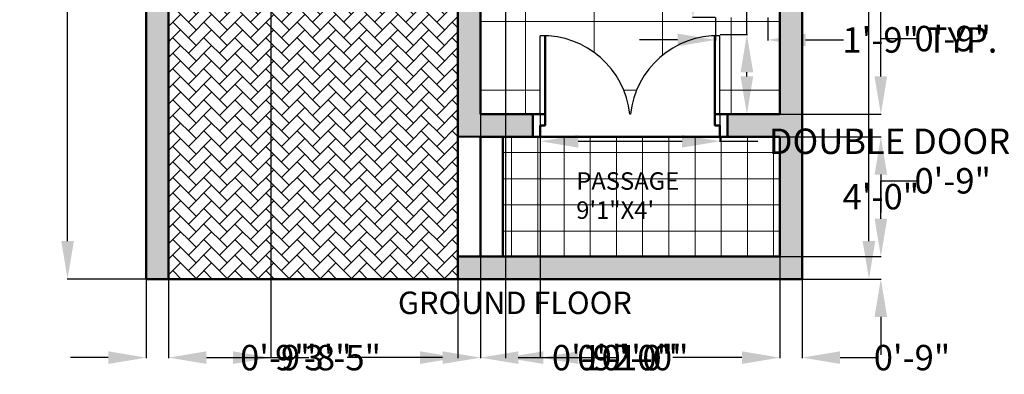
# Model space of a CAD drawing. Units: inches. Extents: x 26 to 14419, y 2 to 3479.
# Tile 1 of 9: x 13608 to 14003, y 2804 to 2946. Entities that reach past the tile are written whole.
import ezdxf

# ---------------------------------------------------------------- set-up
doc = ezdxf.new("R2010")
doc.units = ezdxf.units.IN
doc.header["$MEASUREMENT"] = 0
for name, color, linetype, lineweight in [('A-ANNO-DIMS', 2, 'Continuous', 18), ('A-ANNO-TEXT', 7, 'Continuous', 25), ('A-AREA-IDEN', 7, 'Continuous', 18), ('A-DOOR', 4, 'Continuous', 25), ('A-FLOR-PATT', 252, 'Continuous', 13), ('A-FURN', 8, 'Continuous', 18), ('A-WALL', 7, 'Continuous', 50)]:
    doc.layers.add(name, color=color, linetype=linetype, lineweight=lineweight)
doc.styles.get("Standard").update_dxf_attribs({"font": 'arial.ttf'})
doc.dimstyles.get("Standard").update_dxf_attribs({"dimtxt": 10.18, "dimasz": 15.18, "dimexe": 0.18, "dimexo": 0.0625, "dimgap": 0.09, "dimtad": 0, "dimtih": 1, "dimtoh": 1, "dimdec": 0, "dimzin": 0, "dimdsep": 46, "dimlunit": 3, "dimtxsty": 'Standard', "dimcen": 0.09, "dimadec": 0, "dimazin": 0, "dimtfac": 1, "dimtdec": 0, "dimtofl": 0, "dimtmove": 0, "dimatfit": 3, "dimfxl": 1, "dimtolj": 1, "dimtzin": 0, "dimarcsym": 0})

# ---------------------------------------------------------------- blocks, each defined once
blk = doc.blocks.new('*D7')
at = {"layer": 'A-ANNO-DIMS', "color": 0, "lineweight": -2, "transparency": 16777216}
for p, q in [((13922.15, 3432), (13949, 3432)), ((13948.82, 3416.82), (13948.82, 3142.28)), ((13948.82, 2857.18), (13948.82, 3131.71)), ((13922.15, 2842), (13949, 2842))]:
    blk.add_line(p, q, dxfattribs=at)
at = {"layer": 'A-ANNO-DIMS', "color": 0, "transparency": 16777216}
for points in [[(13946.29, 3416.82), (13951.35, 3416.82), (13948.82, 3432)], [(13946.29, 2857.18), (13951.35, 2857.18), (13948.82, 2842)]]:
    blk.add_solid(points, dxfattribs=at)
at = {"layer": 'Defpoints', "color": 0, "transparency": 16777216}
for p in [(13922.09, 3432), (13922.09, 2842), (13948.82, 2842)]:
    blk.add_point(p, dxfattribs=at)
at = {"layer": 'A-ANNO-DIMS', "color": 0, "transparency": 16777216, "insert": (13948.82, 3137), "char_height": 10.18, "attachment_point": 5}
blk.add_mtext('\\A1;49\'-2"', dxfattribs=at)
blk = doc.blocks.new('DOOR-DOUBLE')
for p, q in [((0, 0), (0, 31.5)), ((72, 0), (72, 31.5)), ((36.16, 0), (35.84, 0))]:
    blk.add_line(p, q)
for centre, start, end in [((1, -3.5), 5.7368, 91.6366), ((71, -3.5), 88.3634, 174.2632)]:
    blk.add_arc(centre, 35.01, start, end)
blk = doc.blocks.new('*D29')
at = {"layer": 'A-ANNO-DIMS', "color": 0, "lineweight": -2, "transparency": 16777216}
for p, q in [((13817.09, 2907.93), (13817.09, 2897.02)), ((13889.09, 2907.93), (13889.09, 2897.02)), ((13832.27, 2897.2), (13873.91, 2897.2)), ((13889.09, 2897.2), (13904.27, 2897.2))]:
    blk.add_line(p, q, dxfattribs=at)
at = {"layer": 'A-ANNO-DIMS', "color": 0, "transparency": 16777216}
for points in [[(13832.27, 2899.73), (13832.27, 2894.67), (13817.09, 2897.2)], [(13873.91, 2899.73), (13873.91, 2894.67), (13889.09, 2897.2)]]:
    blk.add_solid(points, dxfattribs=at)
at = {"layer": 'Defpoints', "color": 0, "transparency": 16777216}
for p in [(13817.09, 2908), (13889.09, 2908), (13889.09, 2897.2)]:
    blk.add_point(p, dxfattribs=at)
at = {"layer": 'A-ANNO-DIMS', "color": 0, "transparency": 16777216, "insert": (13989.66, 2897.2), "char_height": 10.18, "attachment_point": 5}
blk.add_mtext('\\A1;DOUBLE DOOR 6\'-0" TYP.', dxfattribs=at)
blk = doc.blocks.new('*D30')
at = {"layer": 'A-ANNO-DIMS', "color": 0, "lineweight": -2, "transparency": 16777216}
for p, q in [((13899.89, 2940.02), (13899.89, 2955.2)), ((13899.89, 2955.2), (13915.07, 2955.2)), ((13889.15, 2940.02), (13900.07, 2940.02)), ((13899.89, 2923.18), (13899.89, 2924.84)), ((13889.15, 2908), (13900.07, 2908))]:
    blk.add_line(p, q, dxfattribs=at)
at = {"layer": 'A-ANNO-DIMS', "color": 0, "transparency": 16777216}
for points in [[(13897.36, 2924.84), (13902.42, 2924.84), (13899.89, 2940.02)], [(13897.36, 2923.18), (13902.42, 2923.18), (13899.89, 2908)]]:
    blk.add_solid(points, dxfattribs=at)
at = {"layer": 'Defpoints', "color": 0, "transparency": 16777216}
for p in [(13889.09, 2940.02), (13899.89, 2940.02), (13889.09, 2908)]:
    blk.add_point(p, dxfattribs=at)
at = {"layer": 'A-ANNO-DIMS', "color": 0, "transparency": 16777216, "insert": (13946.27, 2955.2), "char_height": 10.18, "attachment_point": 5}
blk.add_mtext('\\A1;2\'-8" TYP.', dxfattribs=at)
blk = doc.blocks.new('*D31')
at = {"layer": 'A-ANNO-DIMS', "color": 0, "lineweight": -2, "transparency": 16777216}
for p, q in [((13887.2, 3006.75), (13878.09, 3006.75)), ((13878.27, 2991.57), (13878.27, 2982.14)), ((13878.27, 2961.99), (13878.27, 2971.42)), ((13887.2, 2946.81), (13878.09, 2946.81))]:
    blk.add_line(p, q, dxfattribs=at)
at = {"layer": 'A-ANNO-DIMS', "color": 0, "transparency": 16777216}
for points in [[(13875.74, 2991.57), (13880.8, 2991.57), (13878.27, 3006.75)], [(13875.74, 2961.99), (13880.8, 2961.99), (13878.27, 2946.81)]]:
    blk.add_solid(points, dxfattribs=at)
at = {"layer": 'Defpoints', "color": 0, "transparency": 16777216}
for p in [(13887.26, 3006.75), (13878.27, 2946.81), (13887.26, 2946.81)]:
    blk.add_point(p, dxfattribs=at)
at = {"layer": 'A-ANNO-DIMS', "color": 0, "transparency": 16777216, "insert": (13878.27, 2976.78), "char_height": 10.18, "attachment_point": 5}
blk.add_mtext('\\A1;3-SEAT SOFA 5\'-0" TYP.', dxfattribs=at)
blk = doc.blocks.new('*D32')
at = {"layer": 'A-ANNO-DIMS', "color": 0, "lineweight": -2, "transparency": 16777216}
for p, q in [((13887.26, 2946.75), (13887.26, 2937.64)), ((13908.25, 2946.75), (13908.25, 2937.64)), ((13872.08, 2937.82), (13856.9, 2937.82)), ((13923.43, 2937.82), (13938.61, 2937.82))]:
    blk.add_line(p, q, dxfattribs=at)
at = {"layer": 'A-ANNO-DIMS', "color": 0, "transparency": 16777216}
for points in [[(13872.08, 2940.35), (13872.08, 2935.29), (13887.26, 2937.82)], [(13923.43, 2940.35), (13923.43, 2935.29), (13908.25, 2937.82)]]:
    blk.add_solid(points, dxfattribs=at)
at = {"layer": 'Defpoints', "color": 0, "transparency": 16777216}
for p in [(13887.26, 2946.81), (13908.25, 2946.81), (13908.25, 2937.82)]:
    blk.add_point(p, dxfattribs=at)
at = {"layer": 'A-ANNO-DIMS', "color": 0, "transparency": 16777216, "insert": (13969.25, 2937.82), "char_height": 10.18, "attachment_point": 5}
blk.add_mtext('\\A1;1\'-9" TYP.', dxfattribs=at)
blk = doc.blocks.new('*D51')
at = {"layer": 'A-ANNO-DIMS', "color": 0, "lineweight": -2, "transparency": 16777216}
for p, q in [((13659.09, 2841.93), (13659.09, 2810.32)), ((13668.09, 2841.93), (13668.09, 2810.32)), ((13643.91, 2810.5), (13628.73, 2810.5)), ((13683.27, 2810.5), (13698.45, 2810.5))]:
    blk.add_line(p, q, dxfattribs=at)
at = {"layer": 'A-ANNO-DIMS', "color": 0, "transparency": 16777216}
for points in [[(13643.91, 2813.03), (13643.91, 2807.97), (13659.09, 2810.5)], [(13683.27, 2813.03), (13683.27, 2807.97), (13668.09, 2810.5)]]:
    blk.add_solid(points, dxfattribs=at)
at = {"layer": 'Defpoints', "color": 0, "transparency": 16777216}
for p in [(13659.09, 2842), (13668.09, 2842), (13668.09, 2810.5)]:
    blk.add_point(p, dxfattribs=at)
at = {"layer": 'A-ANNO-DIMS', "color": 0, "transparency": 16777216, "insert": (13712.07, 2810.5), "char_height": 10.18, "attachment_point": 5}
blk.add_mtext('\\A1;0\'-9"', dxfattribs=at)
blk = doc.blocks.new('*D52')
at = {"layer": 'A-ANNO-DIMS', "color": 0, "lineweight": -2, "transparency": 16777216}
for p, q in [((13668.09, 2841.93), (13668.09, 2810.32)), ((13784.09, 2841.93), (13784.09, 2810.32)), ((13683.27, 2810.5), (13712.47, 2810.5)), ((13768.91, 2810.5), (13739.71, 2810.5))]:
    blk.add_line(p, q, dxfattribs=at)
at = {"layer": 'A-ANNO-DIMS', "color": 0, "transparency": 16777216}
for points in [[(13683.27, 2813.03), (13683.27, 2807.97), (13668.09, 2810.5)], [(13768.91, 2813.03), (13768.91, 2807.97), (13784.09, 2810.5)]]:
    blk.add_solid(points, dxfattribs=at)
at = {"layer": 'Defpoints', "color": 0, "transparency": 16777216}
for p in [(13668.09, 2842), (13784.09, 2842), (13784.09, 2810.5)]:
    blk.add_point(p, dxfattribs=at)
at = {"layer": 'A-ANNO-DIMS', "color": 0, "transparency": 16777216, "insert": (13726.09, 2810.5), "char_height": 10.18, "attachment_point": 5}
blk.add_mtext('\\A1;9\'-8"', dxfattribs=at)
blk = doc.blocks.new('*D53')
at = {"layer": 'A-ANNO-DIMS', "color": 0, "lineweight": -2, "transparency": 16777216}
for p, q in [((13793.09, 2850.93), (13793.09, 2810.32)), ((13784.09, 2841.93), (13784.09, 2810.32)), ((13768.91, 2810.5), (13753.73, 2810.5)), ((13808.27, 2810.5), (13823.45, 2810.5))]:
    blk.add_line(p, q, dxfattribs=at)
at = {"layer": 'A-ANNO-DIMS', "color": 0, "transparency": 16777216}
for points in [[(13768.91, 2813.03), (13768.91, 2807.97), (13784.09, 2810.5)], [(13808.27, 2813.03), (13808.27, 2807.97), (13793.09, 2810.5)]]:
    blk.add_solid(points, dxfattribs=at)
at = {"layer": 'Defpoints', "color": 0, "transparency": 16777216}
for p in [(13793.09, 2851), (13784.09, 2842), (13793.09, 2810.5)]:
    blk.add_point(p, dxfattribs=at)
at = {"layer": 'A-ANNO-DIMS', "color": 0, "transparency": 16777216, "insert": (13837.07, 2810.5), "char_height": 10.18, "attachment_point": 5}
blk.add_mtext('\\A1;0\'-9"', dxfattribs=at)
blk = doc.blocks.new('*D54')
at = {"layer": 'A-ANNO-DIMS', "color": 0, "lineweight": -2, "transparency": 16777216}
for p, q in [((13793.09, 2850.93), (13793.09, 2810.32)), ((13913.09, 2850.93), (13913.09, 2810.32)), ((13808.27, 2810.5), (13836, 2810.5)), ((13897.91, 2810.5), (13870.19, 2810.5))]:
    blk.add_line(p, q, dxfattribs=at)
at = {"layer": 'A-ANNO-DIMS', "color": 0, "transparency": 16777216}
for points in [[(13808.27, 2813.03), (13808.27, 2807.97), (13793.09, 2810.5)], [(13897.91, 2813.03), (13897.91, 2807.97), (13913.09, 2810.5)]]:
    blk.add_solid(points, dxfattribs=at)
at = {"layer": 'Defpoints', "color": 0, "transparency": 16777216}
for p in [(13793.09, 2851), (13913.09, 2851), (13913.09, 2810.5)]:
    blk.add_point(p, dxfattribs=at)
at = {"layer": 'A-ANNO-DIMS', "color": 0, "transparency": 16777216, "insert": (13853.09, 2810.5), "char_height": 10.18, "attachment_point": 5}
blk.add_mtext('\\A1;10\'-0"', dxfattribs=at)
blk = doc.blocks.new('*D55')
at = {"layer": 'A-ANNO-DIMS', "color": 0, "lineweight": -2, "transparency": 16777216}
for p, q in [((13913.09, 2850.93), (13913.09, 2810.32)), ((13922.09, 2841.93), (13922.09, 2810.32)), ((13897.91, 2810.5), (13882.73, 2810.5)), ((13937.27, 2810.5), (13952.45, 2810.5))]:
    blk.add_line(p, q, dxfattribs=at)
at = {"layer": 'A-ANNO-DIMS', "color": 0, "transparency": 16777216}
for points in [[(13897.91, 2813.03), (13897.91, 2807.97), (13913.09, 2810.5)], [(13937.27, 2813.03), (13937.27, 2807.97), (13922.09, 2810.5)]]:
    blk.add_solid(points, dxfattribs=at)
at = {"layer": 'Defpoints', "color": 0, "transparency": 16777216}
for p in [(13913.09, 2851), (13922.09, 2842), (13922.09, 2810.5)]:
    blk.add_point(p, dxfattribs=at)
at = {"layer": 'A-ANNO-DIMS', "color": 0, "transparency": 16777216, "insert": (13966.07, 2810.5), "char_height": 10.18, "attachment_point": 5}
blk.add_mtext('\\A1;0\'-9"', dxfattribs=at)
blk = doc.blocks.new('*D56')
at = {"layer": 'A-ANNO-DIMS', "color": 0, "lineweight": -2, "transparency": 16777216}
for p, q in [((13668.03, 3076), (13627.41, 3076)), ((13627.59, 3060.82), (13627.59, 2964.28)), ((13627.59, 2857.18), (13627.59, 2953.71)), ((13668.03, 2842), (13627.41, 2842))]:
    blk.add_line(p, q, dxfattribs=at)
at = {"layer": 'A-ANNO-DIMS', "color": 0, "transparency": 16777216}
for points in [[(13625.06, 3060.82), (13630.12, 3060.82), (13627.59, 3076)], [(13625.06, 2857.18), (13630.12, 2857.18), (13627.59, 2842)]]:
    blk.add_solid(points, dxfattribs=at)
at = {"layer": 'Defpoints', "color": 0, "transparency": 16777216}
for p in [(13627.59, 3076), (13668.09, 3076), (13668.09, 2842)]:
    blk.add_point(p, dxfattribs=at)
at = {"layer": 'A-ANNO-DIMS', "color": 0, "transparency": 16777216, "insert": (13627.59, 2959), "char_height": 10.18, "attachment_point": 5}
blk.add_mtext('\\A1;19\'-6"', dxfattribs=at)
blk = doc.blocks.new('*D63')
at = {"layer": 'A-ANNO-DIMS', "color": 0, "lineweight": -2, "transparency": 16777216}
for p, q in [((13953.59, 2866.18), (13953.59, 2881.36)), ((13953.59, 2881.36), (13968.77, 2881.36)), ((13913.15, 2851), (13953.77, 2851)), ((13922.15, 2842), (13953.77, 2842)), ((13953.59, 2826.82), (13953.59, 2811.64))]:
    blk.add_line(p, q, dxfattribs=at)
at = {"layer": 'A-ANNO-DIMS', "color": 0, "transparency": 16777216}
for points in [[(13951.06, 2866.18), (13956.12, 2866.18), (13953.59, 2851)], [(13951.06, 2826.82), (13956.12, 2826.82), (13953.59, 2842)]]:
    blk.add_solid(points, dxfattribs=at)
at = {"layer": 'Defpoints', "color": 0, "transparency": 16777216}
for p in [(13913.09, 2851), (13953.59, 2851), (13922.09, 2842)]:
    blk.add_point(p, dxfattribs=at)
at = {"layer": 'A-ANNO-DIMS', "color": 0, "transparency": 16777216, "insert": (13982.39, 2881.36), "char_height": 10.18, "attachment_point": 5}
blk.add_mtext('\\A1;0\'-9"', dxfattribs=at)
blk = doc.blocks.new('*D64')
at = {"layer": 'A-ANNO-DIMS', "color": 0, "lineweight": -2, "transparency": 16777216}
for p, q in [((13913.15, 2899), (13953.77, 2899)), ((13953.59, 2883.82), (13953.59, 2880.28)), ((13953.59, 2866.18), (13953.59, 2869.71)), ((13913.15, 2851), (13953.77, 2851))]:
    blk.add_line(p, q, dxfattribs=at)
at = {"layer": 'A-ANNO-DIMS', "color": 0, "transparency": 16777216}
for points in [[(13951.06, 2883.82), (13956.12, 2883.82), (13953.59, 2899)], [(13951.06, 2866.18), (13956.12, 2866.18), (13953.59, 2851)]]:
    blk.add_solid(points, dxfattribs=at)
at = {"layer": 'Defpoints', "color": 0, "transparency": 16777216}
for p in [(13913.09, 2899), (13953.59, 2899), (13913.09, 2851)]:
    blk.add_point(p, dxfattribs=at)
at = {"layer": 'A-ANNO-DIMS', "color": 0, "transparency": 16777216, "insert": (13953.59, 2875), "char_height": 10.18, "attachment_point": 5}
blk.add_mtext('\\A1;4\'-0"', dxfattribs=at)
blk = doc.blocks.new('*D65')
at = {"layer": 'A-ANNO-DIMS', "color": 0, "lineweight": -2, "transparency": 16777216}
for p, q in [((13953.59, 2923.18), (13953.59, 2938.36)), ((13953.59, 2938.36), (13968.77, 2938.36)), ((13913.15, 2908), (13953.77, 2908)), ((13913.15, 2899), (13953.77, 2899)), ((13953.59, 2883.82), (13953.59, 2868.64))]:
    blk.add_line(p, q, dxfattribs=at)
at = {"layer": 'A-ANNO-DIMS', "color": 0, "transparency": 16777216}
for points in [[(13951.06, 2923.18), (13956.12, 2923.18), (13953.59, 2908)], [(13951.06, 2883.82), (13956.12, 2883.82), (13953.59, 2899)]]:
    blk.add_solid(points, dxfattribs=at)
at = {"layer": 'Defpoints', "color": 0, "transparency": 16777216}
for p in [(13913.09, 2908), (13953.59, 2908), (13913.09, 2899)]:
    blk.add_point(p, dxfattribs=at)
at = {"layer": 'A-ANNO-DIMS', "color": 0, "transparency": 16777216, "insert": (13982.39, 2938.36), "char_height": 10.18, "attachment_point": 5}
blk.add_mtext('\\A1;0\'-9"', dxfattribs=at)
blk = doc.blocks.new('*D66')
at = {"layer": 'A-ANNO-DIMS', "color": 0, "lineweight": -2, "transparency": 16777216}
for p, q in [((13906.22, 3124.24), (13953.77, 3124.24)), ((13953.59, 3109.06), (13953.59, 3021.41)), ((13953.59, 2923.18), (13953.59, 3010.83)), ((13913.15, 2908), (13953.77, 2908))]:
    blk.add_line(p, q, dxfattribs=at)
at = {"layer": 'A-ANNO-DIMS', "color": 0, "transparency": 16777216}
for points in [[(13951.06, 3109.06), (13956.12, 3109.06), (13953.59, 3124.24)], [(13951.06, 2923.18), (13956.12, 2923.18), (13953.59, 2908)]]:
    blk.add_solid(points, dxfattribs=at)
at = {"layer": 'Defpoints', "color": 0, "transparency": 16777216}
for p in [(13906.16, 3124.24), (13953.59, 3124.24), (13913.09, 2908)]:
    blk.add_point(p, dxfattribs=at)
at = {"layer": 'A-ANNO-DIMS', "color": 0, "transparency": 16777216, "insert": (13953.59, 3016.12), "char_height": 10.18, "attachment_point": 5}
blk.add_mtext('\\A1;18\'-0"', dxfattribs=at)
blk = doc.blocks.new('*D73')
at = {"layer": 'A-ANNO-DIMS', "color": 0, "lineweight": -2, "transparency": 16777216}
for p, q in [((13668.09, 3084.93), (13668.09, 2810.32)), ((13709.09, 3084.93), (13709.09, 2810.32)), ((13683.27, 2810.5), (13693.91, 2810.5)), ((13709.09, 2810.5), (13724.27, 2810.5))]:
    blk.add_line(p, q, dxfattribs=at)
at = {"layer": 'A-ANNO-DIMS', "color": 0, "transparency": 16777216}
for points in [[(13683.27, 2813.03), (13683.27, 2807.97), (13668.09, 2810.5)], [(13693.91, 2813.03), (13693.91, 2807.97), (13709.09, 2810.5)]]:
    blk.add_solid(points, dxfattribs=at)
at = {"layer": 'Defpoints', "color": 0, "transparency": 16777216}
for p in [(13668.09, 3085), (13709.09, 3085), (13709.09, 2810.5)]:
    blk.add_point(p, dxfattribs=at)
at = {"layer": 'A-ANNO-DIMS', "color": 0, "transparency": 16777216, "insert": (13737.89, 2810.5), "char_height": 10.18, "attachment_point": 5}
blk.add_mtext('\\A1;3\'-5"', dxfattribs=at)
blk = doc.blocks.new('*D74')
at = {"layer": 'A-ANNO-DIMS', "color": 0, "lineweight": -2, "transparency": 16777216}
for p, q in [((13793.09, 2907.93), (13793.09, 2810.32)), ((13817.09, 2907.93), (13817.09, 2810.32)), ((13777.91, 2810.5), (13762.73, 2810.5)), ((13832.27, 2810.5), (13847.45, 2810.5))]:
    blk.add_line(p, q, dxfattribs=at)
at = {"layer": 'A-ANNO-DIMS', "color": 0, "transparency": 16777216}
for points in [[(13777.91, 2813.03), (13777.91, 2807.97), (13793.09, 2810.5)], [(13832.27, 2813.03), (13832.27, 2807.97), (13817.09, 2810.5)]]:
    blk.add_solid(points, dxfattribs=at)
at = {"layer": 'Defpoints', "color": 0, "transparency": 16777216}
for p in [(13793.09, 2908), (13817.09, 2908), (13817.09, 2810.5)]:
    blk.add_point(p, dxfattribs=at)
at = {"layer": 'A-ANNO-DIMS', "color": 0, "transparency": 16777216, "insert": (13861.16, 2810.5), "char_height": 10.18, "attachment_point": 5}
blk.add_mtext('\\A1;2\'-0"', dxfattribs=at)
blk = doc.blocks.new('*D82')
at = {"layer": 'A-ANNO-DIMS', "color": 0, "lineweight": -2, "transparency": 16777216}
for p, q in [((13793.09, 3126.93), (13793.09, 2810.32)), ((13803.14, 3126.93), (13803.14, 2810.32)), ((13777.91, 2810.5), (13762.73, 2810.5)), ((13818.32, 2810.5), (13833.5, 2810.5))]:
    blk.add_line(p, q, dxfattribs=at)
at = {"layer": 'A-ANNO-DIMS', "color": 0, "transparency": 16777216}
for points in [[(13777.91, 2813.03), (13777.91, 2807.97), (13793.09, 2810.5)], [(13818.32, 2813.03), (13818.32, 2807.97), (13803.14, 2810.5)]]:
    blk.add_solid(points, dxfattribs=at)
at = {"layer": 'Defpoints', "color": 0, "transparency": 16777216}
for p in [(13793.09, 3127), (13803.14, 3127), (13803.14, 2810.5)]:
    blk.add_point(p, dxfattribs=at)
at = {"layer": 'A-ANNO-DIMS', "color": 0, "transparency": 16777216, "insert": (13851.07, 2810.5), "char_height": 10.18, "attachment_point": 5}
blk.add_mtext('\\A1;0\'-10"', dxfattribs=at)

msp = doc.modelspace()

# ---------------------------------------------------------------- hatches: boundary and pattern name
at = {"layer": 'A-FLOR-PATT'}
h = msp.add_hatch(color=256, dxfattribs=at)
h.dxf.hatch_style = 1
h.paths.add_polyline_path([(13922.09, 3432), (13659.09, 3432), (13659.09, 2842), (13668.09, 2842), (13668.09, 2851), (13668.09, 2899), (13668.09, 2908), (13668.09, 3076), (13706.09, 3076), (13706.09, 3085), (13668.09, 3085), (13668.09, 3249), (13712.76, 3249), (13712.76, 3255), (13668.09, 3255), (13668.09, 3375), (13720.94, 3375), (13720.94, 3378, -0.017236), (13720.94, 3380), (13720.94, 3381), (13668.09, 3381), (13668.09, 3423), (13784.09, 3423), (13784.09, 3381), (13753.94, 3381), (13753.94, 3375), (13784.09, 3375), (13784.09, 3255), (13758.77, 3255), (13758.77, 3249), (13784.09, 3249), (13793.09, 3249), (13793.09, 3255), (13793.09, 3423), (13913.09, 3423), (13913.09, 3255), (13832.09, 3255), (13832.09, 3254, -0.014283), (13832.09, 3252), (13832.09, 3249), (13836.57, 3249), (13836.57, 3234), (13839.57, 3234, -0.017236), (13841.57, 3234), (13842.57, 3234), (13842.57, 3249), (13913.09, 3249), (13913.09, 3201), (13892.46, 3201), (13793.09, 3201), (13784.09, 3201), (13784.09, 3195), (13793.09, 3195), (13913.09, 3195), (13913.09, 3127), (13922.09, 3127)])
h.paths.add_polyline_path([(13922.09, 3013.5), (13913.09, 3013.5), (13913.09, 2908), (13892.09, 2908), (13892.09, 2899), (13913.09, 2899), (13913.09, 2851), (13793.09, 2851), (13784.09, 2851), (13784.09, 2842), (13922.09, 2842)], flags=17)
h.paths.add_polyline_path([(13793.09, 3085), (13784.09, 3085), (13784.09, 3076), (13784.09, 3071.08), (13784.09, 3066.17), (13784.09, 2908), (13784.09, 2899.07), (13793.09, 2899), (13802.09, 2899), (13814.09, 2899), (13814.09, 2908), (13793.09, 2908)], flags=17)
h.paths.add_polyline_path([(14342.64, 3401.72), (14242.78, 3401.72), (14242.78, 3392.72), (14257.64, 3392.72), (14257.64, 3351.75), (14257.64, 3345.75), (14257.64, 3330.73), (14263.64, 3330.73), (14263.64, 3392.72), (14333.64, 3392.72), (14333.64, 3284.72), (14302.92, 3284.72), (14302.92, 3281.72, -0.022645), (14302.92, 3279.12), (14302.92, 3278.72), (14333.64, 3278.72), (14333.64, 3170.72), (14316.1, 3170.72), (14263.64, 3170.72), (14263.64, 3278.72), (14269.92, 3278.72), (14269.92, 3284.72), (14263.64, 3284.72), (14257.64, 3284.72), (14257.64, 3225.75), (14257.64, 3219.75), (14257.64, 3164.72), (14333.64, 3164.72), (14333.64, 3110.37), (14210.01, 3110.37), (14210.01, 3104.37), (14257.64, 3104.37), (14257.64, 3024), (14263.64, 3024), (14263.64, 3039.72), (14263.64, 3104.37), (14333.64, 3104.37), (14333.64, 3045.72), (14333.64, 3039.72), (14333.64, 2967.72), (14296.64, 2967.72), (14296.64, 2964.72, -0.017236), (14296.64, 2962.72), (14296.64, 2961.72), (14333.64, 2961.72), (14333.64, 2882.72), (14312.64, 2882.72), (14312.64, 2873.72), (14333.64, 2873.72), (14333.64, 2820.72), (14333.64, 2811.72), (14342.64, 2811.72)])
h.paths.add_polyline_path([(14088.64, 3219.75), (14218.64, 3219.75), (14218.64, 3222.75, -0.014283), (14218.64, 3224.75), (14218.64, 3225.75), (14088.64, 3225.75), (14088.64, 3345.75), (14088.64, 3351.75), (14088.64, 3392.72), (14193.93, 3392.72), (14193.93, 3351.75), (14140.64, 3351.75), (14140.64, 3345.75), (14170.7, 3345.75), (14218.64, 3345.75), (14218.64, 3348.75, -0.014283), (14218.64, 3350.75), (14218.64, 3351.75), (14199.93, 3351.75), (14199.93, 3392.72), (14214.78, 3392.72), (14214.78, 3401.72), (14079.64, 3401.72), (14079.64, 2811.72), (14088.64, 2811.72), (14088.64, 2820.72), (14088.64, 2873.72), (14116.21, 2873.72), (14116.21, 2876.57), (14116.21, 2882.72), (14088.64, 2882.72), (14088.64, 3039.72), (14216.01, 3039.72), (14216.01, 3065.37), (14215.01, 3065.37, -0.014283), (14213.01, 3065.37), (14210.01, 3065.37), (14210.01, 3045.72), (14154.64, 3045.72), (14148.64, 3045.72), (14088.64, 3045.72)])
h.paths.add_polyline_path([(14284.64, 2882.72), (14263.64, 2882.72), (14263.64, 2961.72), (14263.64, 2967.72), (14257.64, 2967.72), (14257.64, 2956.69), (14257.64, 2916.18), (14257.64, 2882.72), (14249.61, 2882.72), (14249.61, 2873.72), (14284.64, 2873.72)], flags=17)
h.paths.add_polyline_path([(14202.78, 2882.72), (14189.55, 2882.72), (14189.55, 2879.95), (14189.55, 2873.72), (14202.78, 2873.72)], flags=17)
h = msp.add_hatch(dxfattribs=at)
h.set_pattern_fill('NET', color=256, scale=220)
h.set_pattern_definition([(0, (61.093, 57.67), (0, 27.5), []), (90, (61.093, 57.67), (-27.5, 2e-15), [])])
h.paths.add_polyline_path([(13913.09, 3127), (13819.09, 3127), (13793.09, 3127), (13784.09, 3127), (13784.09, 3085), (13793.09, 3085), (13793.09, 3040.8), (13806.22, 3040.8), (13806.22, 2983.17), (13793.09, 2983.17), (13793.09, 2908), (13817.09, 2908), (13817.09, 2939.5, -0.393405), (13852.93, 2908), (13853.25, 2908, -0.393405), (13889.09, 2939.5), (13889.09, 2908), (13913.09, 2908)])
h.paths.add_polyline_path([(13878.38, 2997.35), (13878.38, 2965.16), (13858.47, 2965.16), (13858.47, 2997.35)], flags=16)
h.paths.add_polyline_path([(13859.47, 2996.35), (13877.38, 2996.35), (13877.38, 2966.16), (13859.47, 2966.16)], flags=0)
h.paths.add_polyline_path([(13859.41, 3048.61), (13859.41, 3080.81), (13879.32, 3080.81), (13879.32, 3048.61)], flags=16)
h.paths.add_polyline_path([(13860.41, 3049.61), (13860.41, 3079.81), (13878.32, 3079.81), (13878.32, 3049.61)], flags=0)
h.paths.add_polyline_path([(13887.26, 3003.97), (13891.72, 3003.97), (13891.72, 3006.75), (13908.25, 3006.75), (13908.25, 3003.97), (13908.25, 2946.81), (13891.72, 2946.81), (13887.26, 2949.6)], flags=16)
h.paths.add_polyline_path([(13887.26, 3036.93), (13887.26, 3091.3), (13891.72, 3091.3), (13891.72, 3094.09), (13908.25, 3094.09), (13908.25, 3091.3), (13908.25, 3034.14), (13891.72, 3034.14)], flags=16)
h.paths.add_polyline_path([(13893.41, 3027), (13907.93, 3027), (13907.93, 3011.42), (13893.41, 3011.42)], flags=16)
h.paths.add_polyline_path([(13874.64, 3054.21), (13874.87, 3054.49), (13874.86, 3054.52), (13872.61, 3055.96), (13872.7, 3055.53)], flags=0)
h.paths.add_polyline_path([(13873.75, 3054.27), (13874.59, 3055.26), (13872.48, 3056.28), (13872.52, 3055.73), (13872.77, 3055.19), (13873.25, 3054.5)], flags=0)
h.paths.add_polyline_path([(13873.61, 3052.85), (13873.55, 3052.9), (13873.56, 3052.82)], flags=0)
h.paths.add_polyline_path([(13872.76, 3051.79), (13871.09, 3051.54), (13872.51, 3051.58)], flags=0)
h.paths.add_polyline_path([(13894.41, 3026), (13906.93, 3026), (13906.93, 3012.42), (13894.41, 3012.42)], flags=0)
h.paths.add_polyline_path([(13905.32, 2986.18), (13905.32, 3003.97), (13901.96, 3003.97), (13901.96, 2986.18)], flags=0)
h.paths.add_polyline_path([(13901.96, 3073.51), (13905.32, 3073.51), (13905.32, 3091.3), (13901.96, 3091.3)], flags=0)
h.paths.add_polyline_path([(13874.39, 2970.25), (13874.4, 2970.28), (13874.29, 2970.36), (13874.25, 2970.32)], flags=0)
h.paths.add_polyline_path([(13830.89, 3101.09), (13830.89, 3105.55), (13828.1, 3105.55), (13828.1, 3122.08), (13830.89, 3122.08), (13888.05, 3122.08), (13888.05, 3105.55), (13885.26, 3101.09)], flags=16)
h.paths.add_polyline_path([(13848.68, 3115.79), (13848.68, 3119.15), (13830.89, 3119.15), (13830.89, 3115.79)], flags=0)
h.paths.add_polyline_path([(13893.41, 3104.63), (13893.41, 3120.21), (13907.93, 3120.21), (13907.93, 3104.63)], flags=16)
h.paths.add_polyline_path([(13894.41, 3105.63), (13894.41, 3119.21), (13906.93, 3119.21), (13906.93, 3105.63)], flags=0)
h = msp.add_hatch(dxfattribs=at)
h.set_pattern_fill('AR-HBONE', color=256, scale=1.1)
h.set_pattern_definition([(45, (61.093, 57.669), (0, 6.2225397), [13.2, -4.4]), (135, (64.2045, 60.7802), (5e-16, 6.2225397), [13.2, -4.4])])
h.paths.add_polyline_path([(13668.09, 2908), (13668.09, 2899), (13668.09, 2851), (13668.09, 2842), (13784.09, 2842), (13784.09, 2851), (13784.09, 2899), (13784.09, 2908), (13784.09, 3066.17), (13709.09, 3066.17), (13709.09, 3071.08), (13709.09, 3076), (13668.09, 3076)])
h = msp.add_hatch(dxfattribs=at)
h.set_pattern_fill('NET', color=256, scale=84)
h.set_pattern_definition([(0, (61.093, 57.669), (0, 10.5), []), (90, (61.093, 57.669), (-10.5, 6e-16), [])])
h.paths.add_polyline_path([(13817.09, 2899), (13802.09, 2899), (13802.09, 2851), (13913.09, 2851), (13913.09, 2899), (13889.09, 2899)])

# ---------------------------------------------------------------- linework, layer by layer
at = {"layer": 'A-FURN'}
msp.add_lwpolyline([(13793.09, 2842), (13802.09, 2842)], dxfattribs=at)
at = {"layer": 'A-WALL'}
for p, q in [((13659.09, 2842), (13659.09, 3432)), ((13922.09, 3432), (13922.09, 2842)), ((13913.09, 3195), (13913.09, 2908)), ((13793.09, 2908), (13793.09, 3085)), ((13668.09, 2908), (13668.09, 3076)), ((13784.09, 2908), (13784.09, 3076)), ((13819.09, 2903.5), (13819.09, 2939.5)), ((13887.09, 2903.5), (13887.09, 2939.5)), ((13668.09, 2899), (13668.09, 2908)), ((13784.09, 2899), (13784.09, 2908)), ((13819.09, 2908), (13793.09, 2908)), ((13814.09, 2899), (13814.09, 2908)), ((13913.09, 2908), (13887.09, 2908)), ((13892.09, 2899), (13892.09, 2908)), ((13817.09, 2899), (13817.09, 2903.5)), ((13819.09, 2903.5), (13817.09, 2903.5)), ((13887.09, 2903.5), (13889.09, 2903.5)), ((13889.09, 2899), (13889.09, 2903.5)), ((13668.09, 2851), (13668.09, 2899)), ((13793.09, 2899), (13784.09, 2899.07)), ((13784.09, 2851), (13784.09, 2899)), ((13793.09, 2851), (13793.09, 2899)), ((13817.09, 2899), (13793.09, 2899)), ((13817.09, 2899), (13889.09, 2899)), ((13913.09, 2899), (13889.09, 2899)), ((13913.09, 2899), (13913.09, 2851)), ((13668.09, 2851), (13668.09, 2842)), ((13784.09, 2851), (13784.09, 2842)), ((13913.09, 2851), (13793.09, 2851)), ((13668.09, 2842), (13659.09, 2842)), ((13668.09, 2842), (13784.09, 2842)), ((13922.09, 2842), (13784.09, 2842))]:
    msp.add_line(p, q, dxfattribs=at)
for points in [[(13784.09, 2908), (13784.09, 2851), (13793.09, 2851), (13793.09, 2899)], [(13802.09, 2851), (13802.09, 2899), (13793.09, 2899), (13793.09, 2851)]]:
    msp.add_lwpolyline(points, dxfattribs=at)

# ---------------------------------------------------------------- block references
at = {"layer": 'A-DOOR'}
msp.add_blockref('DOOR-DOUBLE', (13817.09, 2908), dxfattribs=at)

# ---------------------------------------------------------------- texts
at = {"layer": 'A-ANNO-TEXT', "insert": (13760.02, 2836.96), "char_height": 9, "attachment_point": 1}
msp.add_mtext_dynamic_manual_height_columns('GROUND FLOOR', width=157.7562, gutter_width=1, heights=[0], dxfattribs=at)
at = {"layer": 'A-AREA-IDEN', "insert": (13831.49, 2884.78), "char_height": 7, "attachment_point": 1}
msp.add_mtext_dynamic_manual_height_columns('PASSAGE\\P9\'1"X4\'', width=51, gutter_width=1, heights=[0], dxfattribs=at)

# ---------------------------------------------------------------- dimensions: what is measured, and where the dimension line sits
at = {"layer": 'A-ANNO-DIMS'}
for base, p1, p2, override, picture, middle in [((13948.82, 2842), (13922.09, 3432), (13922.09, 2842), {"dimclrd": 0, "dimclre": 0, "dimclrt": 0}, '*D7', (13948.82, 3137)), ((13953.59, 3124.24), (13913.09, 2908), (13906.16, 3124.24), {"dimdec": 1, "dimlfac": 1, "dimrnd": 0, "dimzin": 1, "dimdsep": 46, "dimlunit": 4, "dimfrac": 2}, '*D66', (13953.59, 3016.12)), ((13627.59, 3076), (13668.09, 2842), (13668.09, 3076), {"dimdec": 1, "dimlfac": 1, "dimrnd": 0, "dimzin": 1, "dimdsep": 46, "dimlunit": 4, "dimfrac": 2}, '*D56', (13627.59, 2959)), ((13953.59, 2908), (13913.09, 2899), (13913.09, 2908), {"dimdec": 1, "dimlfac": 1, "dimrnd": 0, "dimzin": 1, "dimdsep": 46, "dimlunit": 4, "dimfrac": 2}, '*D65', (13982.39, 2938.36)), ((13953.59, 2899), (13913.09, 2851), (13913.09, 2899), {"dimdec": 1, "dimlfac": 1, "dimrnd": 0, "dimzin": 1, "dimdsep": 46, "dimlunit": 4, "dimfrac": 2}, '*D64', (13953.59, 2875)), ((13953.59, 2851), (13922.09, 2842), (13913.09, 2851), {"dimdec": 1, "dimlfac": 1, "dimrnd": 0, "dimzin": 1, "dimdsep": 46, "dimlunit": 4, "dimfrac": 2}, '*D63', (13982.39, 2881.36))]:
    dim = msp.add_linear_dim(base=base, p1=p1, p2=p2, angle=90, dimstyle='Standard', override=override, dxfattribs=at)
    dim.commit()
    dim.dimension.update_dxf_attribs({"geometry": picture, "text_midpoint": middle})
for base, p1, p2, picture, middle in [((13803.1394, 2810.496), (13793.0912, 3126.996), (13803.1394, 3126.996), '*D82', (13851.0745, 2810.496)), ((13709.09, 2810.5), (13668.09, 3085), (13709.09, 3085), '*D73', (13737.89, 2810.5)), ((13817.09, 2810.5), (13793.09, 2908), (13817.09, 2908), '*D74', (13861.16, 2810.5)), ((13793.09, 2810.5), (13784.09, 2842), (13793.09, 2851), '*D53', (13837.07, 2810.5)), ((13913.09, 2810.5), (13793.09, 2851), (13913.09, 2851), '*D54', (13853.09, 2810.5)), ((13922.09, 2810.5), (13913.09, 2851), (13922.09, 2842), '*D55', (13966.07, 2810.5)), ((13668.09, 2810.5), (13659.09, 2842), (13668.09, 2842), '*D51', (13712.07, 2810.5)), ((13784.09, 2810.5), (13668.09, 2842), (13784.09, 2842), '*D52', (13726.09, 2810.5))]:
    dim = msp.add_linear_dim(base=base, p1=p1, p2=p2, dimstyle='Standard', override={"dimdec": 1, "dimlfac": 1, "dimrnd": 0, "dimzin": 1, "dimdsep": 46, "dimlunit": 4, "dimfrac": 2}, dxfattribs=at)
    dim.commit()
    dim.dimension.update_dxf_attribs({"geometry": picture, "text_midpoint": middle})
for base, p1, p2, angle, text, picture, middle in [((13878.27, 2946.81), (13887.26, 3006.75), (13887.26, 2946.81), 270, '3-SEAT SOFA <> TYP.', '*D31', (13878.27, 2976.78)), ((13899.89, 2940.02), (13889.09, 2908), (13889.09, 2940.02), 90, '<> TYP.', '*D30', (13946.27, 2955.2)), ((13908.25, 2937.82), (13887.26, 2946.81), (13908.25, 2946.81), 0, '<> TYP.', '*D32', (13969.25, 2937.82))]:
    dim = msp.add_linear_dim(base=base, p1=p1, p2=p2, angle=angle, text=text, dimstyle='Standard', override={"dimdec": 1, "dimrnd": 0, "dimzin": 1, "dimlunit": 4, "dimfrac": 2}, dxfattribs=at)
    dim.commit()
    dim.dimension.update_dxf_attribs({"geometry": picture, "text_midpoint": middle})
dim = msp.add_linear_dim(base=(13889.09, 2897.2), p1=(13817.09, 2908), p2=(13889.09, 2908), text='DOUBLE DOOR <> TYP.', dimstyle='Standard', override={"dimdec": 1, "dimrnd": 0, "dimzin": 1, "dimlunit": 4, "dimfrac": 2}, dxfattribs=at)
dim.commit()
dim.dimension.update_dxf_attribs({"geometry": '*D29', "text_midpoint": (13989.66, 2897.2)})

doc.saveas('drawing.dxf')
